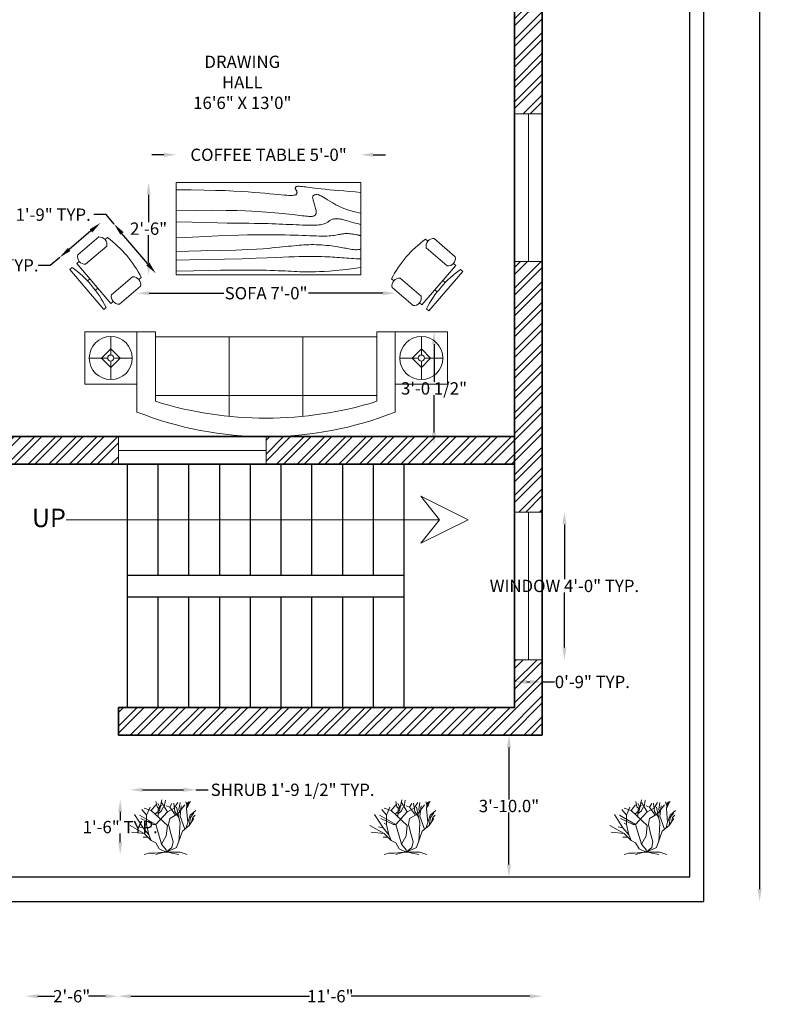
# Model space of a CAD drawing. Units: inches. Extents: x 0 to 478, y -33 to 633.
# Tile 2 of 4: x 234 to 478, y -33 to 286. Entities that reach past the tile are written whole.
import ezdxf

# ---------------------------------------------------------------- set-up
doc = ezdxf.new("R2010")
doc.units = ezdxf.units.IN
for name, color, linetype, lineweight in [('A-ANNO-DIMS', 2, 'Continuous', 18), ('A-ANNO-SYMB', 7, 'Continuous', 18), ('A-ANNO-TEXT', 7, 'Continuous', 18), ('A-AREA-IDEN', 7, 'Continuous', 18), ('A-FLOR-STRS', 7, 'Continuous', 25), ('A-FURN', 8, 'Continuous', 18), ('A-GLAZ', 4, 'Continuous', 18), ('A-WALL', 7, 'Continuous', 35), ('A-WALL-PATT', 252, 'Continuous', 13), ('C-PROP', 7, 'Continuous', 30), ('L-PLNT', 3, 'Continuous', 18)]:
    doc.layers.add(name, color=color, linetype=linetype, lineweight=lineweight)
doc.styles.get("Standard").update_dxf_attribs({"font": 'arial.ttf'})
doc.dimstyles.get("Standard").update_dxf_attribs({"dimtxt": 4, "dimasz": 4, "dimexe": 0.18, "dimexo": 0.0625, "dimgap": 0.09, "dimtad": 0, "dimtih": 1, "dimtoh": 1, "dimdec": 1, "dimzin": 0, "dimdsep": 46, "dimlunit": 3, "dimtxsty": 'Standard', "dimcen": 0.09, "dimse1": 1, "dimse2": 1, "dimadec": 0, "dimazin": 0, "dimtfac": 1, "dimtdec": 1, "dimtofl": 0, "dimtmove": 0, "dimatfit": 3, "dimfxl": 1, "dimtolj": 1, "dimtzin": 0, "dimarcsym": 0})

# ---------------------------------------------------------------- blocks, each defined once
blk = doc.blocks.new('Sofa - Roundback 7 ft.')
for p, q in [((-12.00002, -32.4421), (-12.00003, -6.5971)), ((11.99997, -32.4421), (11.99998, -6.5971)), ((-36.000027, -34), (-36.000027, -11.4696)), ((35.99998, -34), (35.99998, -11.4696)), ((-35.999844, -13.3819), (35.9998, -13.3819)), ((-36.000027, -32.4421), (35.99998, -32.4421))]:
    blk.add_line(p, q)
for points in [[(-36.000027, -34), (-42.000027, -34), (-42.000027, -8)], [(41.99998, -8), (41.99998, -34), (35.99998, -34)]]:
    blk.add_lwpolyline(points)
for centre, radius, start, end in [((0, -114.25), 114.25, 68.43141, 111.5686), ((-0.00001, -127.1968), 121.1968, 72.72033, 107.2797)]:
    blk.add_arc(centre, radius, start, end)
blk = doc.blocks.new('Table - Rectangular Woodgrain 60 x 30 in.')
for p, q in [((0, 0), (0, -30)), ((60, 0), (0, 0)), ((60, -30), (60, 0)), ((0, -30), (60, -30))]:
    blk.add_line(p, q)
for points in [[(0, -2.4), (4.8155, -2.418), (9.0302, -2.4688), (12.709, -2.5477), (15.9167, -2.65), (18.7181, -2.7711), (21.1781, -2.9063), (23.3616, -3.0508), (25.3333, -3.2), (27.1477, -3.3495), (28.8172, -3.4958), (30.3437, -3.636), (31.7291, -3.7667), (32.9756, -3.8849), (34.0849, -3.9875), (35.059, -4.0714), (35.9, -4.1334), (36.6114, -4.1711), (37.2041, -4.1854), (37.6906, -4.1779), (38.0833, -4.15), (38.3948, -4.1034), (38.6375, -4.0396), (38.8239, -3.9602), (38.9666, -3.8667), (39.0764, -3.7608), (39.1573, -3.6448), (39.2116, -3.521), (39.2416, -3.3917), (39.2498, -3.2593), (39.2385, -3.1261), (39.21, -2.9944), (39.1666, -2.8667), (39.111, -2.7447), (39.0468, -2.6281), (38.978, -2.5163), (38.9083, -2.4083), (38.8418, -2.3035), (38.7823, -2.201), (38.7337, -2.1001), (38.7, -2), (38.6844, -1.9003), (38.6875, -1.8021), (38.7094, -1.707), (38.75, -1.6167), (38.8094, -1.5326), (38.8875, -1.4563), (38.9844, -1.3893), (39.1, -1.3333), (39.2351, -1.2896), (39.3937, -1.2583), (39.5804, -1.2396), (39.8, -1.2333), (40.057, -1.2396), (40.3562, -1.2583), (40.7023, -1.2896), (41.1, -1.3333), (41.5547, -1.3895), (42.0755, -1.4573), (42.6721, -1.5361), (43.3542, -1.625), (44.1316, -1.7233), (45.014, -1.8302), (46.0114, -1.9449), (47.1333, -2.0667), (48.3862, -2.1947), (49.7625, -2.3281), (51.2513, -2.4663), (52.8416, -2.6083), (54.5226, -2.7535), (56.2833, -2.9011), (58.1127, -3.0501), (60, -3.2)], [(0, -9.2), (6.5759, -9.0858), (11.9385, -9.0365), (16.2527, -9.0418), (19.6833, -9.0917), (22.3952, -9.1759), (24.5531, -9.2844), (26.322, -9.4069), (27.8666, -9.5333), (29.3241, -9.6553), (30.7203, -9.7719), (32.0532, -9.8837), (33.3208, -9.9917), (34.5213, -10.0965), (35.6526, -10.199), (36.7128, -10.2999), (37.7, -10.4), (38.6129, -10.4996), (39.4531, -10.5969), (40.223, -10.6895), (40.925, -10.775), (41.5613, -10.8512), (42.1344, -10.9156), (42.6465, -10.966), (43.1, -11), (43.4976, -11.0158), (43.8437, -11.0136), (44.143, -10.9942), (44.4, -10.9583), (44.6195, -10.9069), (44.8062, -10.8406), (44.9648, -10.7603), (45.1, -10.6667), (45.2155, -10.5598), (45.3114, -10.4365), (45.3871, -10.2929), (45.4416, -10.125), (45.4743, -9.929), (45.4844, -9.7011), (45.4709, -9.4371), (45.4333, -9.1333), (45.3716, -8.7883), (45.2896, -8.4104), (45.1919, -8.0107), (45.0833, -7.6), (44.9685, -7.1893), (44.8521, -6.7896), (44.7388, -6.4117), (44.6333, -6.0667), (44.54, -5.7628), (44.4614, -5.4979), (44.4001, -5.2675), (44.3583, -5.0667), (44.3384, -4.8909), (44.3427, -4.7354), (44.3736, -4.5956), (44.4333, -4.4667), (44.5236, -4.3453), (44.6427, -4.2333), (44.7884, -4.1339), (44.9583, -4.05), (45.1501, -3.9849), (45.3614, -3.9417), (45.59, -3.9234), (45.8333, -3.9333), (46.0915, -3.9749), (46.3734, -4.0531), (46.6906, -4.1736), (47.0542, -4.3417), (47.4756, -4.5629), (47.9661, -4.8427), (48.5372, -5.1866), (49.2, -5.6), (49.9676, -6.0844), (50.8594, -6.625), (51.8965, -7.2031), (53.1, -7.8), (54.491, -8.3969), (56.0906, -8.975), (57.9199, -9.5156), (60, -10)], [(0, -12.8), (5.1847, -12.9322), (9.6213, -13.0323), (13.3963, -13.1059), (16.5958, -13.1583), (19.3063, -13.1952), (21.614, -13.2219), (23.6054, -13.2439), (25.3666, -13.2667), (26.9728, -13.2947), (28.4531, -13.3281), (29.8256, -13.3663), (31.1083, -13.4083), (32.3191, -13.4535), (33.476, -13.501), (34.597, -13.5501), (35.7, -13.6), (36.7984, -13.6497), (37.8875, -13.6979), (38.9578, -13.743), (40, -13.7833), (41.0047, -13.8174), (41.9625, -13.8438), (42.864, -13.8607), (43.7, -13.8667), (44.4631, -13.8604), (45.1552, -13.8417), (45.7801, -13.8104), (46.3416, -13.7667), (46.8439, -13.7104), (47.2906, -13.6417), (47.6858, -13.5604), (48.0333, -13.4667), (48.3375, -13.3608), (48.6042, -13.2448), (48.8396, -13.121), (49.05, -12.9917), (49.2417, -12.8593), (49.4208, -12.7261), (49.5937, -12.5944), (49.7667, -12.4667), (49.9452, -12.3451), (50.1323, -12.2313), (50.3303, -12.1268), (50.5416, -12.0333), (50.7686, -11.9524), (51.0135, -11.8854), (51.2788, -11.8341), (51.5666, -11.8), (51.8785, -11.7843), (52.2116, -11.7865), (52.562, -11.8059), (52.926, -11.8417), (53.2998, -11.8931), (53.6795, -11.9594), (54.0614, -12.0397), (54.4416, -12.1333), (54.8223, -12.2401), (55.2293, -12.3625), (55.6942, -12.5037), (56.2489, -12.6667), (56.9251, -12.8547), (57.7545, -13.0708), (58.7689, -13.3182), (60, -13.6)], [(0, -18), (5.124, -17.7273), (9.6609, -17.5057), (13.6705, -17.3303), (17.2125, -17.1958), (20.3467, -17.0973), (23.1328, -17.0297), (25.6307, -16.9878), (27.9, -16.9667), (29.9928, -16.9617), (31.9302, -16.9703), (33.7254, -16.9907), (35.3917, -17.0208), (36.9423, -17.0588), (38.3906, -17.1026), (39.7499, -17.1503), (41.0333, -17.2), (42.2519, -17.2496), (43.4073, -17.2969), (44.4986, -17.3395), (45.525, -17.375), (46.4858, -17.4012), (47.3802, -17.4156), (48.2074, -17.416), (48.9667, -17.4), (49.6583, -17.3662), (50.2872, -17.3167), (50.8595, -17.2547), (51.3812, -17.1833), (51.8584, -17.1057), (52.2971, -17.025), (52.7034, -16.9443), (53.0833, -16.8667), (53.443, -16.7951), (53.789, -16.7313), (54.128, -16.6768), (54.4666, -16.6334), (54.8115, -16.6024), (55.1693, -16.5854), (55.5465, -16.5841), (55.95, -16.6), (56.3828, -16.6337), (56.8346, -16.6823), (57.2915, -16.7418), (57.7396, -16.8084), (58.165, -16.878), (58.5539, -16.9469), (58.8924, -17.0111), (59.1666, -17.0667), (59.3679, -17.1107), (59.5078, -17.1438), (59.6032, -17.1675), (59.6708, -17.1833), (59.7275, -17.193), (59.7901, -17.1979), (59.8753, -17.1998), (60, -17.2)], [(0, -22.4), (8.0098, -22.2501), (14.4094, -22.1011), (19.4168, -21.9535), (23.25, -21.8083), (26.1269, -21.6663), (28.2656, -21.5281), (29.884, -21.3947), (31.2, -21.2667), (32.3967, -21.1448), (33.5172, -21.0292), (34.5697, -20.9198), (35.5625, -20.8167), (36.5037, -20.7198), (37.4015, -20.6292), (38.2642, -20.5448), (39.1, -20.4667), (39.9164, -20.3951), (40.7187, -20.3313), (41.5117, -20.2768), (42.3, -20.2333), (43.0883, -20.2024), (43.8812, -20.1854), (44.6836, -20.1841), (45.5, -20.2), (46.3328, -20.234), (47.1747, -20.2844), (48.0163, -20.3488), (48.8479, -20.425), (49.66, -20.5106), (50.4429, -20.6031), (51.1872, -20.7004), (51.8833, -20.8), (52.5246, -20.8999), (53.1166, -20.9995), (53.6681, -21.0983), (54.1875, -21.1958), (54.6834, -21.2919), (55.1646, -21.3859), (55.6394, -21.4777), (56.1167, -21.5667), (56.6028, -21.6515), (57.0961, -21.7266), (57.5929, -21.7852), (58.0896, -21.8208), (58.5823, -21.8268), (59.0674, -21.7964), (59.5412, -21.723), (60, -21.6)], [(0, -25.2), (8.6355, -25.0504), (15.7026, -24.9031), (21.4049, -24.7606), (25.9458, -24.625), (29.529, -24.4988), (32.3578, -24.3844), (34.6359, -24.284), (36.5667, -24.2), (38.3213, -24.1341), (39.9417, -24.0854), (41.437, -24.0523), (42.8167, -24.0333), (44.0901, -24.0268), (45.2667, -24.0313), (46.3557, -24.0451), (47.3667, -24.0667), (48.309, -24.0947), (49.1928, -24.1287), (50.0284, -24.168), (50.826, -24.2125), (51.5959, -24.2617), (52.3483, -24.3151), (53.0935, -24.3725), (53.8417, -24.4334), (54.6009, -24.497), (55.3699, -24.561), (56.1454, -24.6226), (56.9239, -24.6792), (57.7021, -24.7279), (58.4764, -24.7662), (59.2435, -24.7911), (60, -24.8)], [(0, -28.8), (5.6867, -28.6681), (10.45, -28.5698), (14.407, -28.5012), (17.675, -28.4584), (20.3711, -28.4374), (22.6125, -28.4344), (24.5164, -28.4455), (26.2, -28.4667), (27.762, -28.4947), (29.2276, -28.5281), (30.6033, -28.5663), (31.8958, -28.6084), (33.1118, -28.6535), (34.2578, -28.7011), (35.3405, -28.7501), (36.3666, -28.8), (37.3443, -28.8497), (38.288, -28.8974), (39.2137, -28.9412), (40.1375, -28.9792), (41.0753, -29.0093), (42.0432, -29.0297), (43.0572, -29.0384), (44.1333, -29.0333), (45.2936, -29.0114), (46.5843, -28.9641), (48.0579, -28.8816), (49.7666, -28.7542), (51.7629, -28.5721), (54.0989, -28.3255), (56.8272, -28.0048), (60, -27.6)]]:
    blk.add_lwpolyline(points)
blk = doc.blocks.new('Chair - Desk')
for p, q in [((-8.5, 0), (-8.5, -1)), ((-8.5, 0), (8.5, 0)), ((8.5, 0), (8.5, -1)), ((-8.5, -3), (-8.5, -4)), ((-8.5, -3), (8.5, -3)), ((-2, -3), (-2, -1.9355)), ((2, -1.9576), (2, -3)), ((8.5, -3), (8.5, -4)), ((-10.5, -5), (-10.5, -14)), ((-6.5, -14), (-6.5, -5)), ((6.5, -5), (6.5, -14)), ((10.5, -14), (10.5, -5)), ((-8.5, -15), (-8.5, -16)), ((8.5, -15), (8.5, -16))]:
    blk.add_line(p, q)
for centre, radius, start, end in [((0, 34.625), 36.625, 256.5803, 283.4197), ((-8.5, -6.5), 2.5, 36.8699, 143.1301), ((8.5, -6.5), 2.5, 36.8699, 143.1301), ((-8.5, -12.5), 2.5, 216.8699, 323.1301), ((8.5, -12.5), 2.5, 216.8699, 323.1301), ((0, 19.625), 36.625, 256.5803, 283.4197)]:
    blk.add_arc(centre, radius, start, end)
blk = doc.blocks.new('Shrub - elevation')
for p, q in [((-14.88, 18.24), (-12.96, 20.64)), ((-12.471, 19.775), (-12.898, 22.044)), ((-11.28, 19.619), (-12.104, 21.184)), ((-11.433, 18.289), (-10.457, 22.749)), ((-8.16, 17.76), (-10.56, 21.6)), ((-9.48, 19.775), (-8.992, 22.592)), ((-7.2, 19.68), (-6.24, 21.12)), ((-5.086, 17.741), (-5.513, 21.34)), ((-5.28, 19.2), (-3.84, 21.6)), ((-3.84, 16.8), (-0.96, 20.64)), ((-3.377, 18.602), (-2.888, 21.575)), ((-0.508, 21.888), (-0.081, 20.558)), ((-0.203, 19.149), (0.102, 21.34)), ((-0.02, 20.01), (0.896, 21.105)), ((0.041, 20.714), (1.384, 22.044)), ((0.102, 21.34), (0.835, 21.888)), ((-18.24, 11.04), (-21.755, 16.655)), ((-16.8, 16.32), (-18.72, 18.72)), ((-14.88, 18.24), (-17.76, 19.2)), ((-16.8, 16.32), (-15.36, 19.68)), ((-8.16, 12), (-14.88, 18.24)), ((-13.325, 16.724), (-11.433, 18.289)), ((-12.96, 12.48), (-8.16, 17.76)), ((-11.677, 19.071), (-12.471, 19.775)), ((-12.043, 15.628), (-11.921, 18.836)), ((-11.982, 16.802), (-10.579, 18.054)), ((-11.921, 18.836), (-10.64, 20.401)), ((-10.579, 18.054), (-9.846, 19.697)), ((-7.2, 19.68), (-8.64, 20.16)), ((-8.16, 17.76), (-5.28, 19.2)), ((-4.8, 16.32), (-7.2, 19.68)), ((-7.2, 14.88), (-3.84, 16.8)), ((-3.377, 15.315), (-5.086, 17.819)), ((-2.88, 12.96), (-4.32, 19.68)), ((-2.766, 16.802), (-3.377, 18.602)), ((-2.88, 15.84), (-2.4, 20.16)), ((0.346, 13.203), (-0.203, 19.149)), ((-0.142, 19.384), (0.59, 20.401)), ((1.323, 16.254), (3.642, 18.289)), ((1.44, 15.36), (2.88, 17.28)), ((-12.96, 12.48), (-19.68, 16.32)), ((-13.92, 12.48), (-19.2, 14.88)), ((-16.8, 12.48), (-17.76, 12.96)), ((-16.8, 12.48), (-16.8, 16.32)), ((-15.84, 8.16), (-16.8, 12.48)), ((-12.96, 12.48), (-13.92, 12.48)), ((-10.56, 4.32), (-12.96, 12.48)), ((-7.68, 12.48), (-7.2, 14.88)), ((-6.72, 8.64), (-7.68, 12.48)), ((-3.36, 5.28), (-2.88, 12.96)), ((-0.96, 10.56), (-2.88, 15.84)), ((-0.48, 10.8), (0.346, 13.203)), ((0.346, 13.203), (1.323, 16.254)), ((0.96, 12), (1.44, 15.36)), ((0.96, 12), (2.88, 14.88)), ((1.92, 13.44), (2.4, 15.36)), ((2.4, 15.36), (3.36, 16.32)), ((-17.76, 8.64), (-23.663, 11.961)), ((-17.76, 8.64), (-23.128, 9.222)), ((-18.24, 11.04), (-20.16, 11.52)), ((-15.84, 8.16), (-18.24, 11.04)), ((-14.88, 5.76), (-17.76, 8.64)), ((-8.64, 7.68), (-8.16, 12)), ((-5.76, 5.28), (-6.72, 8.64)), ((-4.32, 2.88), (-1.92, 9.6)), ((-1.92, 9.6), (0.96, 12)), ((-16.32, 7.2), (-18.24, 7.2)), ((-14.88, 5.76), (-15.84, 8.16)), ((-12.96, 4.8), (-14.88, 5.76)), ((-11.52, 2.4), (-12.96, 4.8)), ((-10.56, 4.32), (-8.64, 7.68)), ((-8.64, 1.92), (-10.56, 4.32)), ((-6.24, 2.88), (-5.76, 5.28)), ((-15.84, 0.48), (-17.76, 0)), ((-13.44, 0.48), (-15.84, 0.48)), ((-9.6, 0.96), (-13.44, 0.48)), ((-9.6, 0.96), (-12.96, 0)), ((-8.64, 0.96), (-11.52, 2.4)), ((-9.6, 0.96), (-7.68, 0.96)), ((-8.64, 0.96), (-4.32, 2.88)), ((-8.64, 0.96), (-6.24, 2.88)), ((-8.64, 0.96), (-8.64, 1.92)), ((-8.64, 0.96), (-2.88, 0.96)), ((-7.68, 0.96), (-6.24, 0.48)), ((-6.24, 0.48), (-3.36, 0)), ((-2.88, 0.96), (0, 0))]:
    blk.add_line(p, q)
blk = doc.blocks.new('*D20')
at = {"layer": 'A-ANNO-DIMS', "color": 0, "lineweight": -2, "transparency": 16777216}
for p, q in [((392.67, 50), (392.67, 33.13)), ((392.67, 12), (392.67, 28.87))]:
    blk.add_line(p, q, dxfattribs=at)
at = {"layer": 'A-ANNO-DIMS', "color": 0, "transparency": 16777216}
for points in [[(392, 50), (393.34, 50), (392.67, 54)], [(392, 12), (393.34, 12), (392.67, 8)]]:
    blk.add_solid(points, dxfattribs=at)
at = {"layer": 'Defpoints', "color": 0, "transparency": 16777216}
for p in [(403.5, 54), (392.67, 8), (403.5, 8)]:
    blk.add_point(p, dxfattribs=at)
at = {"layer": 'A-ANNO-DIMS', "color": 0, "transparency": 16777216, "insert": (392.67, 31), "char_height": 4, "attachment_point": 5}
blk.add_mtext('\\A1;3\'-10.0"', dxfattribs=at)
blk = doc.blocks.new('*D24')
at = {"layer": 'A-ANNO-DIMS', "color": 0, "lineweight": -2, "transparency": 16777216}
for p, q in [((474.18, 596), (474.18, 302.13)), ((474.18, 4), (474.18, 297.87))]:
    blk.add_line(p, q, dxfattribs=at)
at = {"layer": 'A-ANNO-DIMS', "color": 0, "transparency": 16777216}
for points in [[(473.51, 596), (474.84, 596), (474.18, 600)], [(473.51, 4), (474.84, 4), (474.18, 0)]]:
    blk.add_solid(points, dxfattribs=at)
at = {"layer": 'Defpoints', "color": 0, "transparency": 16777216}
for p in [(456, 600), (474.18, 600), (456, 0)]:
    blk.add_point(p, dxfattribs=at)
at = {"layer": 'A-ANNO-DIMS', "color": 0, "transparency": 16777216, "insert": (474.18, 300), "char_height": 4, "attachment_point": 5}
blk.add_mtext("\\A1;50'", dxfattribs=at)
blk = doc.blocks.new('WIN-48IN')
for p, q in [((0, 48), (9, 48)), ((4.5, 48), (4.5, 0)), ((0, 0), (9, 0))]:
    blk.add_line(p, q)
blk = doc.blocks.new('Lamp - Table')
for p, q in [((0, 7), (0, 1)), ((-1, 0), (-7, 0)), ((0, 3), (-3, 0)), ((-3, 0), (0, -3)), ((3, 0), (0, 3)), ((0, -3), (3, 0)), ((1, 0), (7, 0)), ((0, -1), (0, -7))]:
    blk.add_line(p, q)
for radius in [7, 1]:
    blk.add_circle((0, 0), radius)
blk = doc.blocks.new('END-TABLE-WITH-LAMP')
blk.add_lwpolyline([(-8.49, 8.49), (-8.49, -8.49), (8.49, -8.49), (8.49, 8.49)], close=True)
blk.add_blockref('Lamp - Table', (0, 0))
blk = doc.blocks.new('*D30')
at = {"layer": 'A-ANNO-DIMS', "color": 0, "lineweight": -2, "transparency": 16777216}
for p, q in [((273.48, 36.26), (286.84, 36.26)), ((290.84, 36.26), (294.84, 36.26))]:
    blk.add_line(p, q, dxfattribs=at)
at = {"layer": 'A-ANNO-DIMS', "color": 0, "transparency": 16777216}
for points in [[(273.48, 36.93), (273.48, 35.6), (269.48, 36.26)], [(286.84, 36.93), (286.84, 35.6), (290.84, 36.26)]]:
    blk.add_solid(points, dxfattribs=at)
at = {"layer": 'Defpoints', "color": 0, "transparency": 16777216}
for p in [(290.84, 36.26), (269.48, 33.06), (290.84, 33.06)]:
    blk.add_point(p, dxfattribs=at)
at = {"layer": 'A-ANNO-DIMS', "color": 0, "transparency": 16777216, "insert": (322.33, 36.26), "char_height": 4, "attachment_point": 5}
blk.add_mtext('\\A1;SHRUB 1\'-9 1/2" TYP.', dxfattribs=at)
blk = doc.blocks.new('*D31')
at = {"layer": 'A-ANNO-DIMS', "color": 0, "lineweight": -2, "transparency": 16777216}
for p, q in [((266.27, 29.06), (266.27, 26.29)), ((266.27, 19.26), (266.27, 22.03))]:
    blk.add_line(p, q, dxfattribs=at)
at = {"layer": 'A-ANNO-DIMS', "color": 0, "transparency": 16777216}
for points in [[(265.61, 29.06), (266.94, 29.06), (266.27, 33.06)], [(265.61, 19.26), (266.94, 19.26), (266.27, 15.26)]]:
    blk.add_solid(points, dxfattribs=at)
at = {"layer": 'Defpoints', "color": 0, "transparency": 16777216}
for p in [(266.27, 33.06), (269.48, 33.06), (269.48, 15.26)]:
    blk.add_point(p, dxfattribs=at)
at = {"layer": 'A-ANNO-DIMS', "color": 0, "transparency": 16777216, "insert": (266.27, 24.16), "char_height": 4, "attachment_point": 5}
blk.add_mtext('\\A1;1\'-6" TYP.', dxfattribs=at)
blk = doc.blocks.new('*D34')
at = {"layer": 'A-ANNO-DIMS', "color": 0, "lineweight": -2, "transparency": 16777216}
for p, q in [((410.7, 122.5), (410.7, 104.66)), ((410.7, 82.5), (410.7, 100.34))]:
    blk.add_line(p, q, dxfattribs=at)
at = {"layer": 'A-ANNO-DIMS', "color": 0, "transparency": 16777216}
for points in [[(410.03, 122.5), (411.37, 122.5), (410.7, 126.5)], [(410.03, 82.5), (411.37, 82.5), (410.7, 78.5)]]:
    blk.add_solid(points, dxfattribs=at)
at = {"layer": 'Defpoints', "color": 0, "transparency": 16777216}
for p in [(403.5, 126.5), (410.7, 126.5), (403.5, 78.5)]:
    blk.add_point(p, dxfattribs=at)
at = {"layer": 'A-ANNO-DIMS', "color": 0, "transparency": 16777216, "insert": (410.7, 102.5), "char_height": 4, "attachment_point": 5}
blk.add_mtext('\\A1;WINDOW 4\'-0" TYP.', dxfattribs=at)
blk = doc.blocks.new('*D35')
at = {"layer": 'A-ANNO-DIMS', "color": 0, "lineweight": -2, "transparency": 16777216}
for p, q in [((398.5, 71.3), (399.5, 71.3)), ((403.5, 71.3), (407.5, 71.3))]:
    blk.add_line(p, q, dxfattribs=at)
at = {"layer": 'A-ANNO-DIMS', "color": 0, "transparency": 16777216}
for points in [[(398.5, 71.97), (398.5, 70.63), (394.5, 71.3)], [(399.5, 71.97), (399.5, 70.63), (403.5, 71.3)]]:
    blk.add_solid(points, dxfattribs=at)
at = {"layer": 'Defpoints', "color": 0, "transparency": 16777216}
for p in [(394.5, 78.5), (403.5, 78.5), (403.5, 71.3)]:
    blk.add_point(p, dxfattribs=at)
at = {"layer": 'A-ANNO-DIMS', "color": 0, "transparency": 16777216, "insert": (419.78, 71.3), "char_height": 4, "attachment_point": 5}
blk.add_mtext('\\A1;0\'-9" TYP.', dxfattribs=at)
blk = doc.blocks.new('*D44')
at = {"layer": 'A-ANNO-DIMS', "color": 0, "lineweight": -2, "transparency": 16777216}
for p, q in [((261.68, 223.12), (257.68, 223.12)), ((264.27, 220.07), (261.68, 223.12)), ((275.25, 207.09), (266.85, 217.01))]:
    blk.add_line(p, q, dxfattribs=at)
at = {"layer": 'A-ANNO-DIMS', "color": 0, "transparency": 16777216}
for points in [[(267.36, 217.44), (266.34, 216.58), (264.27, 220.07)], [(275.76, 207.53), (274.74, 206.66), (277.84, 204.04)]]:
    blk.add_solid(points, dxfattribs=at)
at = {"layer": 'Defpoints', "color": 0, "transparency": 16777216}
for p in [(261.86, 218.03), (264.27, 220.07), (275.43, 202.01)]:
    blk.add_point(p, dxfattribs=at)
at = {"layer": 'A-ANNO-DIMS', "color": 0, "transparency": 16777216, "insert": (235.95, 223.12), "char_height": 4, "attachment_point": 5}
blk.add_mtext('\\A1;CHAIR 1\'-9" TYP.', dxfattribs=at)
blk = doc.blocks.new('*D45')
at = {"layer": 'A-ANNO-DIMS', "color": 0, "lineweight": -2, "transparency": 16777216}
for p, q in [((256.77, 217.85), (249.65, 211.82)), ((246.6, 209.23), (243.55, 206.65)), ((243.55, 206.65), (239.55, 206.65))]:
    blk.add_line(p, q, dxfattribs=at)
at = {"layer": 'A-ANNO-DIMS', "color": 0, "transparency": 16777216}
for points in [[(256.34, 218.36), (257.2, 217.34), (259.83, 220.43)], [(249.22, 212.32), (250.08, 211.31), (246.6, 209.23)]]:
    blk.add_solid(points, dxfattribs=at)
at = {"layer": 'Defpoints', "color": 0, "transparency": 16777216}
for p in [(261.86, 218.03), (246.6, 209.23), (248.64, 206.83)]:
    blk.add_point(p, dxfattribs=at)
at = {"layer": 'A-ANNO-DIMS', "color": 0, "transparency": 16777216, "insert": (222.79, 206.65), "char_height": 4, "attachment_point": 5}
blk.add_mtext('\\A1;1\'-5 1/2" TYP.', dxfattribs=at)
blk = doc.blocks.new('*D48')
at = {"layer": 'A-ANNO-DIMS', "color": 0, "lineweight": -2, "transparency": 16777216}
for p, q in [((275.7, 197.6), (299.92, 197.6)), ((351.7, 197.6), (327.48, 197.6))]:
    blk.add_line(p, q, dxfattribs=at)
at = {"layer": 'A-ANNO-DIMS', "color": 0, "transparency": 16777216}
for points in [[(275.7, 198.27), (275.7, 196.93), (271.7, 197.6)], [(351.7, 198.27), (351.7, 196.93), (355.7, 197.6)]]:
    blk.add_solid(points, dxfattribs=at)
at = {"layer": 'Defpoints', "color": 0, "transparency": 16777216}
for p in [(355.7, 197.6), (271.7, 185), (355.7, 185)]:
    blk.add_point(p, dxfattribs=at)
at = {"layer": 'A-ANNO-DIMS', "color": 0, "transparency": 16777216, "insert": (313.7, 197.6), "char_height": 4, "attachment_point": 5}
blk.add_mtext('\\A1;SOFA 7\'-0"', dxfattribs=at)
blk = doc.blocks.new('*D49')
at = {"layer": 'A-ANNO-DIMS', "color": 0, "lineweight": -2, "transparency": 16777216}
for p, q in [((368.3, 181), (368.3, 168.83)), ((368.3, 152.33), (368.3, 164.51))]:
    blk.add_line(p, q, dxfattribs=at)
at = {"layer": 'A-ANNO-DIMS', "color": 0, "transparency": 16777216}
for points in [[(367.63, 181), (368.97, 181), (368.3, 185)], [(367.63, 152.33), (368.97, 152.33), (368.3, 148.33)]]:
    blk.add_solid(points, dxfattribs=at)
at = {"layer": 'Defpoints', "color": 0, "transparency": 16777216}
for p in [(355.7, 185), (355.7, 148.33), (368.3, 148.33)]:
    blk.add_point(p, dxfattribs=at)
at = {"layer": 'A-ANNO-DIMS', "color": 0, "transparency": 16777216, "insert": (368.3, 166.67), "char_height": 4, "attachment_point": 5}
blk.add_mtext('\\A1;3\'-0 1/2"', dxfattribs=at)
blk = doc.blocks.new('*D50')
at = {"layer": 'A-ANNO-DIMS', "color": 0, "lineweight": -2, "transparency": 16777216}
for p, q in [((280.5, 242.56), (276.5, 242.56)), ((348.5, 242.56), (352.5, 242.56))]:
    blk.add_line(p, q, dxfattribs=at)
at = {"layer": 'A-ANNO-DIMS', "color": 0, "transparency": 16777216}
for points in [[(280.5, 243.23), (280.5, 241.89), (284.5, 242.56)], [(348.5, 243.23), (348.5, 241.89), (344.5, 242.56)]]:
    blk.add_solid(points, dxfattribs=at)
at = {"layer": 'Defpoints', "color": 0, "transparency": 16777216}
for p in [(344.5, 242.56), (284.5, 233.56), (344.5, 233.56)]:
    blk.add_point(p, dxfattribs=at)
at = {"layer": 'A-ANNO-DIMS', "color": 0, "transparency": 16777216, "insert": (314.5, 242.56), "char_height": 4, "attachment_point": 5}
blk.add_mtext('\\A1;COFFEE TABLE 5\'-0"', dxfattribs=at)
blk = doc.blocks.new('*D51')
at = {"layer": 'A-ANNO-DIMS', "color": 0, "lineweight": -2, "transparency": 16777216}
for p, q in [((275.5, 229.56), (275.5, 220.69)), ((275.5, 207.56), (275.5, 216.43))]:
    blk.add_line(p, q, dxfattribs=at)
at = {"layer": 'A-ANNO-DIMS', "color": 0, "transparency": 16777216}
for points in [[(274.84, 229.56), (276.17, 229.56), (275.5, 233.56)], [(274.84, 207.56), (276.17, 207.56), (275.5, 203.56)]]:
    blk.add_solid(points, dxfattribs=at)
at = {"layer": 'Defpoints', "color": 0, "transparency": 16777216}
for p in [(275.5, 233.56), (284.5, 233.56), (284.5, 203.56)]:
    blk.add_point(p, dxfattribs=at)
at = {"layer": 'A-ANNO-DIMS', "color": 0, "transparency": 16777216, "insert": (275.5, 218.56), "char_height": 4, "attachment_point": 5}
blk.add_mtext('\\A1;2\'-6"', dxfattribs=at)
blk = doc.blocks.new('*D54')
at = {"layer": 'A-ANNO-DIMS', "color": 0, "lineweight": -2, "transparency": 16777216}
for p, q in [((269.7, -30.8), (327.83, -30.8)), ((399.5, -30.8), (341.37, -30.8))]:
    blk.add_line(p, q, dxfattribs=at)
at = {"layer": 'A-ANNO-DIMS', "color": 0, "transparency": 16777216}
for points in [[(269.7, -30.13), (269.7, -31.47), (265.7, -30.8)], [(399.5, -30.13), (399.5, -31.47), (403.5, -30.8)]]:
    blk.add_solid(points, dxfattribs=at)
at = {"layer": 'Defpoints', "color": 0, "transparency": 16777216}
for p in [(265.7, 54), (403.5, 54), (403.5, -30.8)]:
    blk.add_point(p, dxfattribs=at)
at = {"layer": 'A-ANNO-DIMS', "color": 0, "transparency": 16777216, "insert": (334.6, -30.8), "char_height": 4, "attachment_point": 5}
blk.add_mtext('\\A1;11\'-6"', dxfattribs=at)
blk = doc.blocks.new('*D57')
at = {"layer": 'A-ANNO-DIMS', "color": 0, "lineweight": -2, "transparency": 16777216}
for p, q in [((239.5, -30.8), (245.06, -30.8)), ((261.5, -30.8), (255.94, -30.8))]:
    blk.add_line(p, q, dxfattribs=at)
at = {"layer": 'A-ANNO-DIMS', "color": 0, "transparency": 16777216}
for points in [[(239.5, -30.13), (239.5, -31.47), (235.5, -30.8)], [(261.5, -30.13), (261.5, -31.47), (265.5, -30.8)]]:
    blk.add_solid(points, dxfattribs=at)
at = {"layer": 'Defpoints', "color": 0, "transparency": 16777216}
for p in [(235.5, 448.5), (265.5, 448.5), (265.5, -30.8)]:
    blk.add_point(p, dxfattribs=at)
at = {"layer": 'A-ANNO-DIMS', "color": 0, "transparency": 16777216, "insert": (250.5, -30.8), "char_height": 4, "attachment_point": 5}
blk.add_mtext('\\A1;2\'-6"', dxfattribs=at)

msp = doc.modelspace()

# ---------------------------------------------------------------- hatches: boundary and pattern name
at = {"layer": 'A-WALL-PATT'}
h = msp.add_hatch(dxfattribs=at)
h.set_pattern_fill('ANSI32', color=256, scale=0.5)
h.paths.add_polyline_path([(456, 600), (45, 600), (45, 547.04), (54, 547.04), (54, 591), (447, 591), (447, 507), (433.5, 507), (433.5, 498), (456, 498)])
h.paths.add_polyline_path([(54, 499.04), (45, 499.04), (45, 429), (54, 429)])
h.paths.add_polyline_path([(235.5, 453), (226.5, 453), (226.5, 591), (222, 591), (222, 453), (213, 453), (213, 448.5), (235.5, 448.5)])
h.paths.add_polyline_path([(105, 453), (54, 453), (54, 448.5), (105, 448.5)], flags=17)
h.paths.add_polyline_path([(183, 453), (129, 453), (129, 448.5), (138, 448.5), (138, 388.5), (54, 388.5), (54, 384), (138, 384), (138, 324), (129, 324), (129, 319.5), (192, 319.5), (192, 310.5), (196.5, 310.5), (196.5, 324), (142.5, 324), (142.5, 448.5), (183, 448.5)])
h.paths.add_polyline_path([(403.5, 453), (265.5, 453), (265.5, 448.5), (394.5, 448.5), (394.5, 442.5), (397.5, 442.5), (403.5, 442.5)])
h.paths.add_polyline_path([(412.5, 507), (399, 507), (399, 558), (394.5, 558), (394.5, 498), (412.5, 498)], flags=17)
h.paths.add_polyline_path([(399, 591), (394.5, 591), (394.5, 582), (399, 582)], flags=17)
h.paths.add_polyline_path([(54, 408), (45, 408), (45, 364.5), (54, 364.5)])
h.paths.add_polyline_path([(54, 343.5), (45, 343.5), (45, 275.82), (54, 275.82), (54, 319.5)])
h.paths.add_polyline_path([(105, 324), (54, 324), (54, 319.5), (105, 319.5)], flags=17)
h.paths.add_polyline_path([(403.5, 412.5), (397.5, 412.5), (394.5, 412.5), (394.5, 388.53), (403.5, 388.53)])
h.paths.add_polyline_path([(403.5, 340.53), (394.5, 340.53), (394.5, 311.5), (256.5, 311.5), (256.5, 307), (394.5, 307), (394.5, 255.85), (403.5, 255.85)])
h.paths.add_polyline_path([(54, 216.47), (54, 227.82), (45, 227.82), (45, 190.5), (95.47, 190.5), (95.47, 199.5), (70.97, 199.5), (54, 199.5)])
h.paths.add_polyline_path([(196.5, 280.5), (192, 280.5), (192, 199.5), (143.47, 199.5), (143.47, 190.5), (187.5, 190.5), (187.5, 188.75), (193.5, 188.75), (196.5, 188.75)])
h.paths.add_polyline_path([(403.5, 207.85), (394.5, 207.85), (394.5, 126.5), (403.5, 126.5)])
h.paths.add_polyline_path([(403.5, 78.5), (394.5, 78.5), (394.5, 63), (265.7, 63), (265.7, 54), (403.5, 54)])
h.paths.add_polyline_path([(394.5, 151), (313.7, 151), (313.7, 142), (394.5, 142)])
h.paths.add_polyline_path([(265.7, 151), (196.5, 151), (196.5, 152.75), (193.5, 152.75), (187.5, 152.75), (187.5, 142), (265.7, 142)])

# ---------------------------------------------------------------- linework, layer by layer
at = {"layer": 'A-ANNO-SYMB'}
msp.add_line((248.73, 124), (370.03, 124), dxfattribs=at)
msp.add_lwpolyline([(370.03, 124), (364.05, 116.39), (379.35, 124), (364.05, 131.61)], close=True, dxfattribs=at)
at = {"layer": 'A-FLOR-STRS'}
for p, q in [((268.5, 142), (268.5, 63)), ((278.5, 142), (278.5, 106)), ((288.5, 142), (288.5, 106)), ((298.5, 142), (298.5, 106)), ((308.5, 142), (308.5, 106)), ((318.5, 142), (318.5, 106)), ((328.5, 142), (328.5, 106)), ((338.5, 142), (338.5, 106)), ((348.5, 142), (348.5, 106)), ((358.5, 142), (358.5, 63)), ((394.5, 142), (394.5, 63)), ((268.5, 106), (358.5, 106)), ((268.5, 99), (358.5, 99)), ((278.5, 99), (278.5, 63)), ((288.5, 99), (288.5, 63)), ((298.5, 99), (298.5, 63)), ((308.5, 99), (308.5, 63)), ((318.5, 99), (318.5, 63)), ((328.5, 99), (328.5, 63)), ((338.5, 99), (338.5, 63)), ((348.5, 99), (348.5, 63))]:
    msp.add_line(p, q, dxfattribs=at)
at = {"layer": 'A-WALL'}
for p, q in [((403.5, 54), (403.5, 412.5)), ((394.5, 63), (394.5, 307)), ((394.5, 151), (196.5, 151)), ((394.5, 142), (187.5, 142)), ((265.7, 63), (394.5, 63)), ((265.7, 63), (265.7, 54)), ((265.7, 54), (403.5, 54))]:
    msp.add_line(p, q, dxfattribs=at)
at = {"layer": 'C-PROP'}
for p, q in [((456, 0), (456, 600)), ((451.5, 8), (451.5, 498)), ((8, 8), (451.5, 8)), ((0, 0), (456, 0))]:
    msp.add_line(p, q, dxfattribs=at)

# ---------------------------------------------------------------- block references
at = {"layer": 'A-FURN'}
for name, p in [('Table - Rectangular Woodgrain 60 x 30 in.', (284.5, 233.56)), ('END-TABLE-WITH-LAMP', (263.21, 176.51))]:
    msp.add_blockref(name, p, dxfattribs=at)
at = {"layer": 'A-FURN', "rotation": 130.2661944961201}
msp.add_blockref('Chair - Desk', (255.42, 198.82), dxfattribs=at)
at = {"layer": 'A-FURN', "xscale": -1, "rotation": 229.1783506366166}
msp.add_blockref('Chair - Desk', (372.12, 198.25), dxfattribs=at)
at = {"layer": 'A-FURN', "extrusion": (0, 1e-16, -1), "rotation": 180}
msp.add_blockref('Sofa - Roundback 7 ft.', (-313.7, 151), dxfattribs=at)
at = {"layer": 'A-FURN', "extrusion": (0, 0, -1), "zscale": -1}
msp.add_blockref('END-TABLE-WITH-LAMP', (-364.18, 176.51), dxfattribs=at)
at = {"layer": 'A-GLAZ'}
for p in [(394.5, 207.85), (394.5, 78.5)]:
    msp.add_blockref('WIN-48IN', p, dxfattribs=at)
at = {"layer": 'A-GLAZ', "rotation": 269.9999999999999}
msp.add_blockref('WIN-48IN', (265.7, 151), dxfattribs=at)
at = {"layer": 'L-PLNT', "xscale": 0.78234725202095, "yscale": 0.78234725202095, "zscale": 0.78234725202095}
for p in [(287.99, 15.26), (365.99, 15.26), (443.99, 15.26)]:
    msp.add_blockref('Shrub - elevation', p, dxfattribs=at)

# ---------------------------------------------------------------- texts
at = {"layer": 'A-ANNO-TEXT', "insert": (237.53, 127.6), "char_height": 6, "attachment_point": 1}
msp.add_mtext_dynamic_manual_height_columns('UP', width=13.1294, gutter_width=12.5, heights=[0], dxfattribs=at)
at = {"layer": 'A-AREA-IDEN', "ltscale": 0.5, "insert": (287.09, 274.77), "char_height": 4, "attachment_point": 1}
msp.add_mtext_dynamic_manual_height_columns('\\pxqc;DRAWING HALL\\P16\'6" X 13\'0"', width=37.7397, gutter_width=12.5, heights=[0], dxfattribs=at)

# ---------------------------------------------------------------- dimensions: what is measured, and where the dimension line sits
at = {"layer": 'A-ANNO-DIMS'}
for base, p1, p2, angle, override, picture, middle in [((474.18, 600), (456, 0), (456, 600), 90, {"dimclrd": 0, "dimclre": 0, "dimclrt": 0}, '*D24', (474.18, 300)), ((275.5, 233.56), (284.5, 203.56), (284.5, 233.56), 90, {"dimdec": 1, "dimlfac": 1, "dimrnd": 0, "dimzin": 1, "dimdsep": 46, "dimlunit": 4, "dimfrac": 2}, '*D51', (275.5, 218.56)), ((368.3, 148.33), (355.7, 185), (355.7, 148.33), 270, {"dimdec": 1, "dimlfac": 1, "dimrnd": 0, "dimzin": 1, "dimdsep": 46, "dimlunit": 4, "dimfrac": 2}, '*D49', (368.3, 166.67)), ((392.67, 8), (403.5, 54), (403.5, 8), 90, {"dimclrd": 0, "dimclre": 0, "dimclrt": 0}, '*D20', (392.67, 31))]:
    dim = msp.add_linear_dim(base=base, p1=p1, p2=p2, angle=angle, dimstyle='Standard', override=override, dxfattribs=at)
    dim.commit()
    dim.dimension.update_dxf_attribs({"geometry": picture, "text_midpoint": middle})
for base, p1, p2, picture, middle in [((265.5, -30.8), (235.5, 448.5), (265.5, 448.5), '*D57', (250.5, -30.8)), ((403.5, -30.8), (265.7, 54), (403.5, 54), '*D54', (334.6, -30.8))]:
    dim = msp.add_linear_dim(base=base, p1=p1, p2=p2, dimstyle='Standard', override={"dimdec": 1, "dimlfac": 1, "dimrnd": 0, "dimzin": 1, "dimdsep": 46, "dimlunit": 4, "dimfrac": 2}, dxfattribs=at)
    dim.commit()
    dim.dimension.update_dxf_attribs({"geometry": picture, "text_midpoint": middle})
for base, p1, p2, text, picture, middle in [((344.5, 242.56), (284.5, 233.56), (344.5, 233.56), 'COFFEE TABLE <>', '*D50', (314.5, 242.56)), ((355.7, 197.6), (271.7, 185), (355.7, 185), 'SOFA <>', '*D48', (313.7, 197.6)), ((403.5, 71.3), (394.5, 78.5), (403.5, 78.5), '<> TYP.', '*D35', (419.78, 71.3)), ((290.84, 36.26), (269.48, 33.06), (290.84, 33.06), 'SHRUB <> TYP.', '*D30', (322.33, 36.26))]:
    dim = msp.add_linear_dim(base=base, p1=p1, p2=p2, text=text, dimstyle='Standard', override={"dimdec": 1, "dimlfac": 1, "dimrnd": 0, "dimzin": 1, "dimdsep": 46, "dimlunit": 4, "dimfrac": 2}, dxfattribs=at)
    dim.commit()
    dim.dimension.update_dxf_attribs({"geometry": picture, "text_midpoint": middle})
for base, p1, p2, angle, text, picture, middle in [((264.27, 220.07), (275.43, 202.01), (261.86, 218.03), 130.2662, 'CHAIR <> TYP.', '*D44', (235.95, 223.12)), ((246.6, 209.23), (261.86, 218.03), (248.64, 206.83), 220.2662, '<> TYP.', '*D45', (222.79, 206.65)), ((410.7, 126.5), (403.5, 78.5), (403.5, 126.5), 90, 'WINDOW <> TYP.', '*D34', (410.7, 102.5)), ((266.27, 33.06), (269.48, 15.26), (269.48, 33.06), 90, '<> TYP.', '*D31', (266.27, 24.16))]:
    dim = msp.add_linear_dim(base=base, p1=p1, p2=p2, angle=angle, text=text, dimstyle='Standard', override={"dimdec": 1, "dimlfac": 1, "dimrnd": 0, "dimzin": 1, "dimdsep": 46, "dimlunit": 4, "dimfrac": 2}, dxfattribs=at)
    dim.commit()
    dim.dimension.update_dxf_attribs({"geometry": picture, "text_midpoint": middle})

doc.saveas('drawing.dxf')
